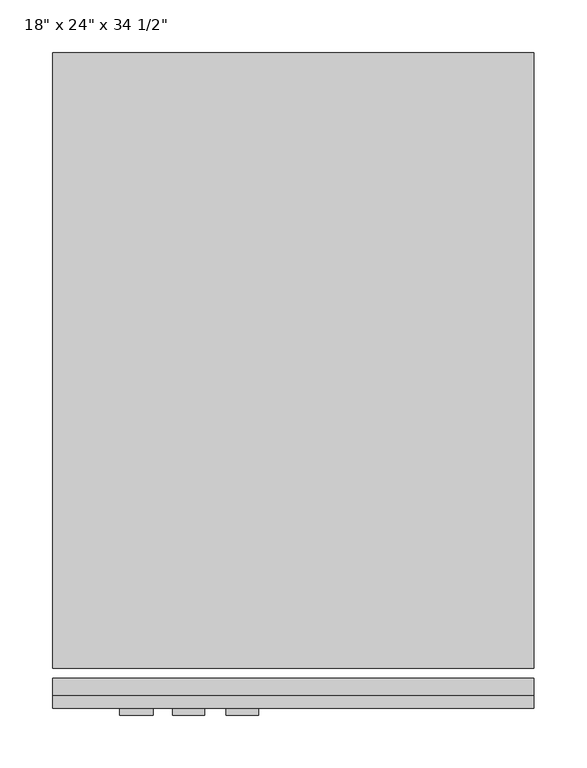
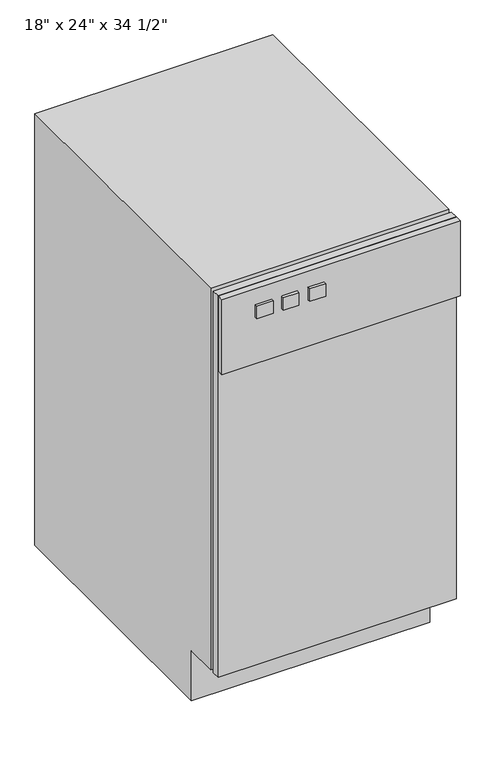
"""IFC4 building model written with IfcOpenShell, lengths in millimetres: proxy geometry."""

from ifc_helpers import new_model, si_unit, frame, origin, place, context, project, spatial, polyline, outline, extrude, source, transform, mapped, element, save


def proxy_7e1014cc(model_context):
    return source(origin(), model_context, "Body", "SweptSolid", [
        extrude(outline(polyline([(534.7174685, -38.3504352), (77.5174685, -38.3504352), (77.5174685, -22.4754352), (534.7174685, -22.4754352), (534.7174685, -38.3504352)])), frame((0.0, 0.0, 101.6), z_axis=(0.0, 0.0, 1.0), x_axis=(1.0, 0.0, 0.0)), (0.0, 0.0, 1.0), 774.7),
        extrude(outline(polyline([(534.7174685, -38.3504352), (534.7174685, -51.0504352), (77.5174685, -51.0504352), (77.5174685, -38.3504352), (534.7174685, -38.3504352)])), frame((0.0, 0.0, 723.9), z_axis=(0.0, 0.0, 1.0), x_axis=(1.0, 0.0, 0.0)), (0.0, 0.0, 1.0), 152.4),
        extrude(outline(polyline([(571.2495648, 0.0), (50.5495648, 0.0), (50.5495648, 101.6), (-12.9504352, 101.6), (-12.9504352, 876.3), (571.2495648, 876.3), (571.2495648, 0.0)])), frame((77.5174685, 0.0, 0.0), z_axis=(1.0, 0.0, 0.0), x_axis=(0.0, 1.0, 0.0)), (0.0, 0.0, 1.0), 457.2),
        extrude(outline(polyline([(172.7674685, -57.4004352), (141.0174685, -57.4004352), (141.0174685, -51.0504352), (172.7674685, -51.0504352), (172.7674685, -57.4004352)])), frame((0.0, 0.0, 818.6415009), z_axis=(0.0, 0.0, 1.0), x_axis=(1.0, 0.0, 0.0)), (0.0, 0.0, 1.0), 25.4),
        extrude(outline(polyline([(221.6847918, -57.4004352), (191.3389562, -57.4004352), (191.3389562, -51.0504352), (221.6847918, -51.0504352), (221.6847918, -57.4004352)])), frame((0.0, 0.0, 818.6415009), z_axis=(0.0, 0.0, 1.0), x_axis=(1.0, 0.0, 0.0)), (0.0, 0.0, 1.0), 25.4),
        extrude(outline(polyline([(272.969254, -57.4004352), (242.3199601, -57.4004352), (242.3199601, -51.0504352), (272.969254, -51.0504352), (272.969254, -57.4004352)])), frame((0.0, 0.0, 818.6415009), z_axis=(0.0, 0.0, 1.0), x_axis=(1.0, 0.0, 0.0)), (0.0, 0.0, 1.0), 25.4),
    ])


if __name__ == "__main__":
    model = new_model("IFC4")
    model_context = context("Model", 3, world=origin())
    ifc_project = project(units=[si_unit("LENGTHUNIT", "METRE", prefix="MILLI")], contexts=[model_context])
    site = spatial("IfcSite", under=ifc_project)
    building = spatial("IfcBuilding", under=site)
    placement = place(None, origin())
    proxy_shape = proxy_7e1014cc(model_context)
    element("IfcBuildingElementProxy", 1, Name="18\" x 24\" x 34 1/2\"", ObjectType="18\" x 24\" x 34 1/2\"", at=placement, inside=building, context=model_context, shape_type="MappedRepresentation", body=[
        mapped(proxy_shape, transform((0.0, 0.0, 0.0), x_axis=(1.0, 0.0, 0.0), y_axis=(0.0, 1.0, 0.0), z_axis=(0.0, 0.0, 1.0))),
    ])
    save(model, "model.ifc")

# Revit data of these elements
# Type "18\" x 24\" x 34 1/2\""
#   Label = "T"
#   Assembly Code = "E1090400"
#   Depth = 2' - 0"
#   Height = 2' - 10 1/2"
#   Width = 1' - 6"
#   Panel Face Material = Plastic, Opaque Black
#   Trach Compact. Material = Steel, Paint Finish, Ivory, Matte
#   Default Elevation = 0
# Element 1 (IfcBuildingElementProxy, "18\" x 24\" x 34 1/2\"")
#   Materials on its faces: "Steel, Paint Finish, Ivory, Matte", "Plastic, Opaque Black"
# Materials
#   "Plastic, Opaque Black": class "Plastic", colour RGB 0 0 0, transparency 0.7, Description = "Plastic, generic, opaque black", Cost = 0
#   "Steel, Paint Finish, Ivory, Matte": class "Metal", colour RGB 247 247 239, transparency 0, Description = "Steel, paint finish, ivory, matte", Cost = 0
